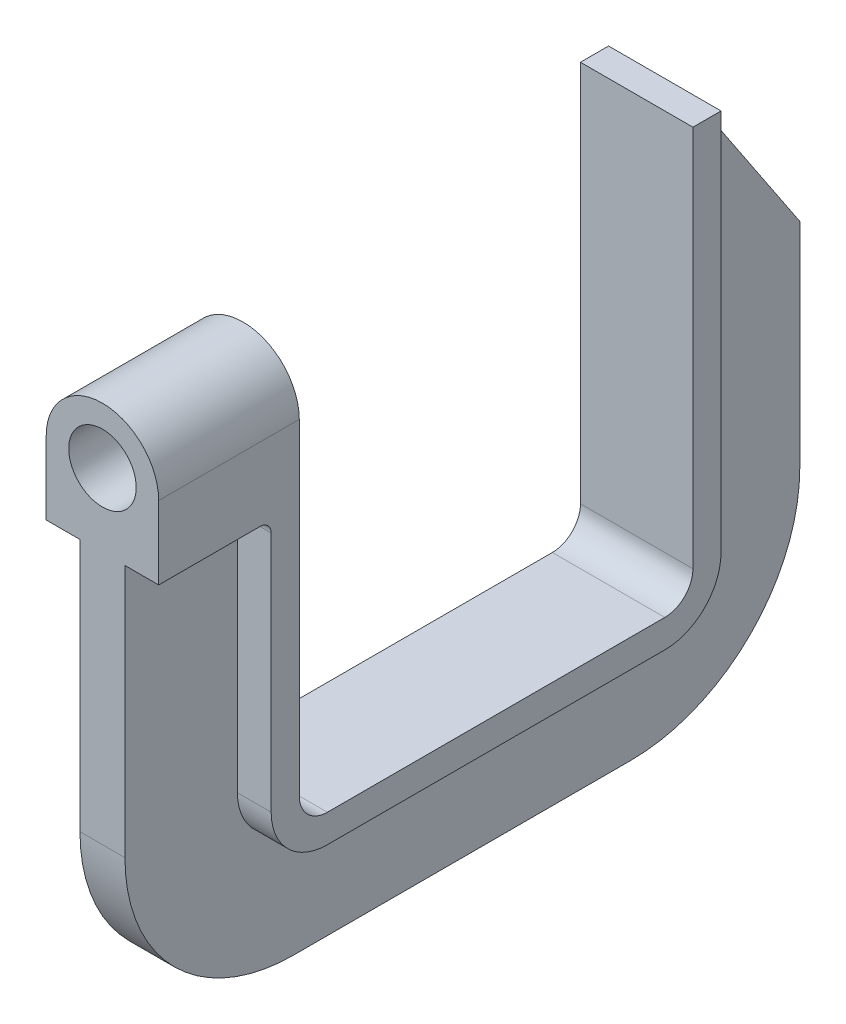
SolidWorks part; units mm, degrees
material "Plain Carbon Steel"
ref_plane "Front Plane" through (0, 0, 0) normal (0, 0, 1) x (1, 0, 0)
ref_plane "Top Plane" through (0, 0, 0) normal (0, 1, 0) x (1, 0, 0)
ref_plane "Right Plane" through (0, 0, 0) normal (1, 0, 0) x (0, 0, -1)
sketch "C-Frame Profile Sketch" plane through (0, 0, 0) normal (1, 0, 0) x (0, 0, -1)
  line L0 (-854.8584, 0) -> (41888.0628, 0) construction
  line L1 (0, -854.8584) -> (0, 41888.0628) construction
  line L2 (0, 75) -> (0, 30)
  line L3 (30, 0) -> (90, 0)
  line L4 (120, 30) -> (120, 68)
  line L5 (120, 68) -> (100, 98)
  line L7 (0, 75) -> (25, 75)
  line L8 (25, 75) -> (25, 30)
  line L12 (30, 25) -> (90, 25)
  line L13 (95, 30) -> (95, 98)
  line L14 (95, 98) -> (100, 98)
  arc A0 (90, 25) -> (95, 30) centre (90, 30) ccw
  arc A1 (90, 0) -> (120, 30) centre (90, 30) ccw
  arc A2 (0, 30) -> (30, 0) centre (30, 30) ccw
  arc A3 (30, 25) -> (25, 30) centre (30, 30) cw
  point P18 (120, 0)
  point P22 (0, 0)
  dimension "D7" = 5
  dimension "D8" = 30
  dimension "D9" = 30
  dimension "D10" = 5
  dimension "D1" = 75
  dimension "D2" = 68
  dimension "D3" = 30
  dimension "D4" = 120
  dimension "D5" = 5
  dimension "D6" = 70
extrude "C-Frame Body" add sketch "C-Frame Profile Sketch" along normal mid plane 8
sketch "Frame Rim Sketch" plane through (0, 0, 0) normal (1, 0, 0) x (0, 0, -1)
  line L0 (25, 75) -> (20, 75)
  line L1 (20, 75) -> (20, 30)
  line L2 (25, 75) -> (25, 30)
  line L3 (30, 25) -> (90, 25)
  line L4 (95, 30) -> (95, 98)
  line L5 (95, 98) -> (100, 98)
  line L6 (100, 98) -> (100, 30)
  line L7 (90, 20) -> (30, 20)
  line L8 (90, 25) -> (30, 25) construction
  arc A0 (25, 30) -> (30, 25) centre (30, 30) ccw
  arc A1 (95, 30) -> (90, 25) centre (90, 30) cw
  arc A2 (30, 20) -> (20, 30) centre (30, 30) cw
  arc A3 (100, 30) -> (90, 20) centre (90, 30) cw
  dimension "D3" = 5
  dimension "D4" = 5
  dimension "D5" = 10
  dimension "D6" = 10
  dimension "D1" = 5
  dimension "D2" = 5
extrude "Frame Rim" add sketch "Frame Rim Sketch" along normal mid plane 20
sketch "Screw Boss Sketch" plane through (0, 0, 0) normal (0, 0, 1) x (1, 0, 0)
  line L0 (-10, 75) -> (10, 75)
  line L1 (10, 75) -> (10, 88)
  line L2 (10, 98) -> (10, 30) construction
  line L3 (-10, 98) -> (-10, 30) construction
  line L4 (-10, 88) -> (-10, 75)
  line L5 (10, 98) -> (-10, 98) construction
  arc A0 (10, 88) -> (-10, 88) centre (0, 88) ccw
  point P13 (0, 98)
  point P14 (0, 98)
extrude "Screw Boss" add sketch "Screw Boss Sketch" against normal blind 25
sketch "Screw Bore Sketch" plane through (0, 0, 0) normal (0, 0, 1) x (1, 0, 0)
  circle A0 centre (0, 88) radius 6
  dimension "D1" = 12
extrude "Screw Bore Ø12" cut sketch "Screw Bore Sketch" against normal blind 43
fillet "Edge Fillets R2" radius 2 2 edges at (-7, 75, -20) (7, 75, -20)
